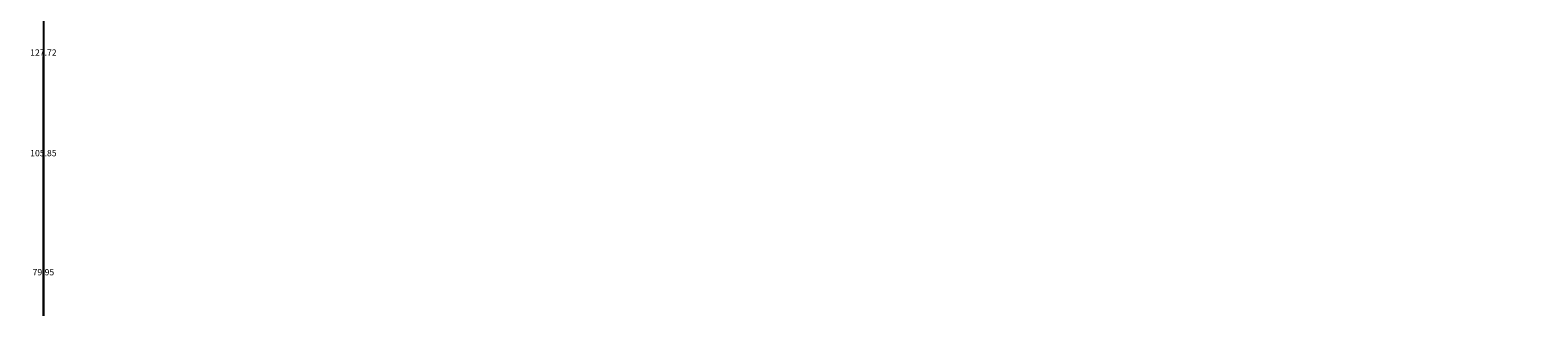
# Model space of a CAD drawing. Units: inches. Extents: x -145 to 510, y 5 to 386.
# Tile 8 of 25: x -145 to 18, y 236 to 266. Entities that reach past the tile are written whole.
import ezdxf

# ---------------------------------------------------------------- set-up
doc = ezdxf.new("R2010")
doc.units = ezdxf.units.IN
doc.header["$MEASUREMENT"] = 0
doc.layers.add('A-ANNO-DIMS', color=2, linetype='Continuous', lineweight=18)
doc.styles.get("Standard").update_dxf_attribs({"font": 'arial.ttf'})
doc.dimstyles.get("Standard").update_dxf_attribs({"dimtxt": 0.6875, "dimasz": 0.18, "dimexe": 0.18, "dimexo": 0.0625, "dimgap": 0.09, "dimtad": 0, "dimtih": 1, "dimtoh": 1, "dimdec": 4, "dimzin": 0, "dimdsep": 46, "dimlunit": 4, "dimtxsty": 'Standard', "dimcen": 0.09, "dimadec": 0, "dimazin": 0, "dimtfac": 1, "dimtdec": 4, "dimtofl": 0, "dimtmove": 0, "dimatfit": 3, "dimfxl": 1, "dimtolj": 1, "dimtzin": 0, "dimarcsym": 0})

# ---------------------------------------------------------------- blocks, each defined once
blk = doc.blocks.new('*D19')
at = {"layer": 'A-ANNO-DIMS', "color": 0, "lineweight": -2, "transparency": 16777216}
for p, q in [((478.76, 355.89), (-144.05, 355.89)), ((-143.87, 355.71), (-143.87, 218.33)), ((-143.87, 80.07), (-143.87, 217.45)), ((-114.04, 79.89), (-144.05, 79.89))]:
    blk.add_line(p, q, dxfattribs=at)
at = {"layer": 'A-ANNO-DIMS', "color": 0, "transparency": 16777216}
for points in [[(-143.9, 355.71), (-143.84, 355.71), (-143.87, 355.89)], [(-143.9, 80.07), (-143.84, 80.07), (-143.87, 79.89)]]:
    blk.add_solid(points, dxfattribs=at)
at = {"layer": 'Defpoints', "color": 0, "transparency": 16777216}
for p in [(-143.87, 355.89), (478.83, 355.89), (-113.97, 79.89)]:
    blk.add_point(p, dxfattribs=at)
at = {"layer": 'A-ANNO-DIMS', "color": 0, "transparency": 16777216, "insert": (-143.87, 217.89), "char_height": 0.688, "attachment_point": 5}
blk.add_mtext('\\A1;276', dxfattribs=at)
blk = doc.blocks.new('*D21')
at = {"layer": 'A-ANNO-DIMS', "color": 0, "lineweight": -2, "transparency": 16777216}
for p, q in [((34.21, 327.61), (-144.05, 327.61)), ((-143.87, 327.43), (-143.87, 264.19)), ((-143.87, 200.07), (-143.87, 263.31)), ((69.71, 199.89), (-144.05, 199.89))]:
    blk.add_line(p, q, dxfattribs=at)
at = {"layer": 'A-ANNO-DIMS', "color": 0, "transparency": 16777216}
for points in [[(-143.9, 327.43), (-143.84, 327.43), (-143.87, 327.61)], [(-143.9, 200.07), (-143.84, 200.07), (-143.87, 199.89)]]:
    blk.add_solid(points, dxfattribs=at)
at = {"layer": 'Defpoints', "color": 0, "transparency": 16777216}
for p in [(-143.87, 327.61), (34.27, 327.61), (69.78, 199.89)]:
    blk.add_point(p, dxfattribs=at)
at = {"layer": 'A-ANNO-DIMS', "color": 0, "transparency": 16777216, "insert": (-143.87, 263.75), "char_height": 0.688, "attachment_point": 5}
blk.add_mtext('\\A1;127.72', dxfattribs=at)
blk = doc.blocks.new('*D26')
at = {"layer": 'A-ANNO-DIMS', "color": 0, "lineweight": -2, "transparency": 16777216}
for p, q in [((95.08, 305.74), (-144.05, 305.74)), ((-143.87, 305.56), (-143.87, 253.26)), ((-143.87, 200.07), (-143.87, 252.38)), ((95.08, 199.89), (-144.05, 199.89))]:
    blk.add_line(p, q, dxfattribs=at)
at = {"layer": 'A-ANNO-DIMS', "color": 0, "transparency": 16777216}
for points in [[(-143.9, 305.56), (-143.84, 305.56), (-143.87, 305.74)], [(-143.9, 200.07), (-143.84, 200.07), (-143.87, 199.89)]]:
    blk.add_solid(points, dxfattribs=at)
at = {"layer": 'Defpoints', "color": 0, "transparency": 16777216}
for p in [(-143.87, 305.74), (95.14, 305.74), (95.14, 199.89)]:
    blk.add_point(p, dxfattribs=at)
at = {"layer": 'A-ANNO-DIMS', "color": 0, "transparency": 16777216, "insert": (-143.87, 252.82), "char_height": 0.688, "attachment_point": 5}
blk.add_mtext('\\A1;105.85', dxfattribs=at)
blk = doc.blocks.new('*D27')
at = {"layer": 'A-ANNO-DIMS', "color": 0, "lineweight": -2, "transparency": 16777216}
for p, q in [((244.23, 279.84), (-144.05, 279.84)), ((-143.87, 279.66), (-143.87, 240.31)), ((-143.87, 200.07), (-143.87, 239.43)), ((218.29, 199.89), (-144.05, 199.89))]:
    blk.add_line(p, q, dxfattribs=at)
at = {"layer": 'A-ANNO-DIMS', "color": 0, "transparency": 16777216}
for points in [[(-143.9, 279.66), (-143.84, 279.66), (-143.87, 279.84)], [(-143.9, 200.07), (-143.84, 200.07), (-143.87, 199.89)]]:
    blk.add_solid(points, dxfattribs=at)
at = {"layer": 'Defpoints', "color": 0, "transparency": 16777216}
for p in [(-143.87, 279.84), (244.29, 279.84), (218.36, 199.89)]:
    blk.add_point(p, dxfattribs=at)
at = {"layer": 'A-ANNO-DIMS', "color": 0, "transparency": 16777216, "insert": (-143.87, 239.87), "char_height": 0.688, "attachment_point": 5}
blk.add_mtext('\\A1;79.95', dxfattribs=at)

msp = doc.modelspace()

# ---------------------------------------------------------------- dimensions: what is measured, and where the dimension line sits
at = {"layer": 'A-ANNO-DIMS'}
for base, p1, p2, override, picture, middle in [((-143.8737, 355.8905), (-113.9737, 79.8905), (478.8263, 355.8905), {"dimdec": 0, "dimlfac": 1, "dimrnd": 0, "dimzin": 0, "dimdsep": 46, "dimlunit": 2}, '*D19', (-143.8737, 217.8905)), ((-143.8737, 327.6093), (69.7763, 199.8905), (34.2706, 327.6093), {"dimdec": 2, "dimlfac": 1, "dimrnd": 0, "dimzin": 0, "dimdsep": 46, "dimlunit": 2}, '*D21', (-143.8737, 263.7499)), ((-143.8737, 305.7416), (95.1414, 199.8905), (95.1414, 305.7416), {"dimdec": 2, "dimlfac": 1, "dimrnd": 0, "dimzin": 0, "dimdsep": 46, "dimlunit": 2}, '*D26', (-143.8737, 252.8161)), ((-143.8737, 279.8443), (218.3571, 199.8905), (244.2916, 279.8443), {"dimdec": 2, "dimlfac": 1, "dimrnd": 0, "dimzin": 0, "dimdsep": 46, "dimlunit": 2}, '*D27', (-143.8737, 239.8674))]:
    dim = msp.add_linear_dim(base=base, p1=p1, p2=p2, angle=90, dimstyle='Standard', override=override, dxfattribs=at)
    dim.commit()
    dim.dimension.update_dxf_attribs({"geometry": picture, "text_midpoint": middle})

doc.saveas('drawing.dxf')
